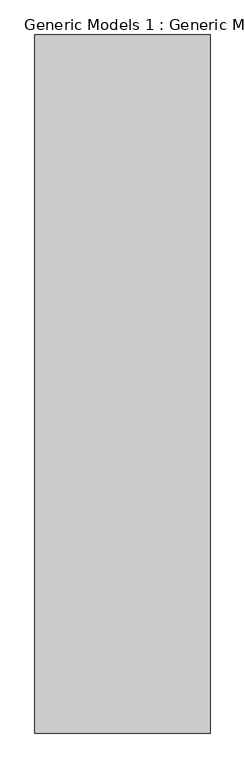
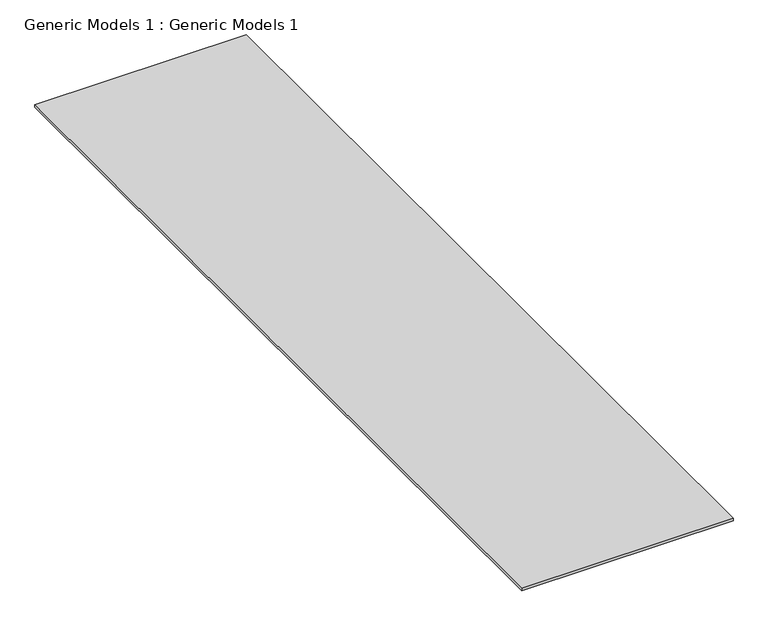
"""IFC4 building model written with IfcOpenShell, lengths in millimetres: proxy geometry, Generic Models 1 : Generic Models 1."""

from ifc_helpers import new_model, si_unit, origin, origin_with_axes, place, context, project, spatial, polyline, outline, extrude, source, transform, mapped, element, save


def generic_models_1_generic_models_1_dbe57743(model_context):
    return source(origin(), model_context, "Body", "SweptSolid", [
        extrude(outline(polyline([(32339.2494112, 30560.4007204), (32339.2494112, -14246.4628995), (21097.8872949, -14246.4628995), (21097.8872949, 30560.4007204), (32339.2494112, 30560.4007204)])), origin_with_axes(), (0.0, 0.0, 1.0), 127.164319),
    ])


if __name__ == "__main__":
    model = new_model("IFC4")
    model_context = context("Model", 3, world=origin())
    ifc_project = project(units=[si_unit("LENGTHUNIT", "METRE", prefix="MILLI")], contexts=[model_context])
    site = spatial("IfcSite", under=ifc_project)
    building = spatial("IfcBuilding", under=site)
    placement = place(None, origin())
    generic_models_1_generic_models_1_shape = generic_models_1_generic_models_1_dbe57743(model_context)
    element("IfcBuildingElementProxy", 1, Name="Generic Models 1 : Generic Models 1", ObjectType="Generic Models 1 : Generic Models 1", at=placement, inside=building, context=model_context, shape_type="MappedRepresentation", body=[
        mapped(generic_models_1_generic_models_1_shape, transform((0.0, 0.0, 0.0), x_axis=(1.0, 0.0, 0.0), y_axis=(0.0, 1.0, 0.0), z_axis=(0.0, 0.0, 1.0))),
    ])
    save(model, "model.ifc")
